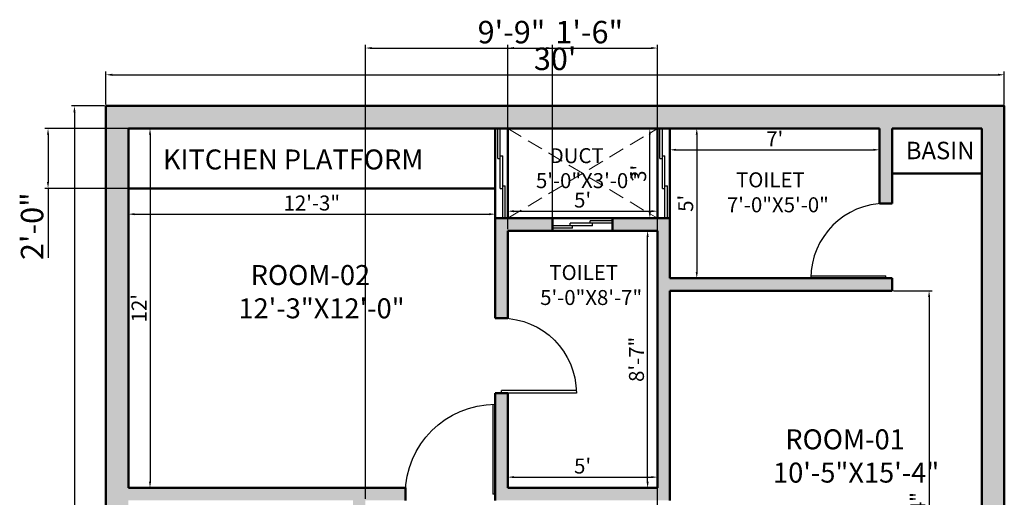
# Model space of a CAD drawing. Units: inches. Extents: x 3274 to 5176, y 1085 to 2172.
# Tile 4 of 16: x 3763 to 4158, y 1383 to 1574. Entities that reach past the tile are written whole.
import ezdxf

# ---------------------------------------------------------------- set-up
doc = ezdxf.new("R2010")
doc.units = ezdxf.units.IN
doc.linetypes.add('DASHED', pattern=[19.05, 12.7, -6.35])
for name, color, linetype, lineweight in [('A-ANNO-DIMS', 2, 'Continuous', 18), ('A-AREA-IDEN', 3, 'Continuous', 25), ('A-DOOR', 4, 'Continuous', 25), ('A-FLOR-OPEN', 7, 'DASHED', 18), ('A-GLAZ', 5, 'Continuous', 25), ('A-WALL', 7, 'Continuous', 50), ('A-WALL-PATT', 8, 'Continuous', 13)]:
    doc.layers.add(name, color=color, linetype=linetype, lineweight=lineweight)
doc.styles.get("Standard").update_dxf_attribs({"font": 'arial.ttf'})
doc.dimstyles.new('ISO-25', dxfattribs={"dimtxt": 9, "dimasz": 2.5, "dimexe": 1.25, "dimexo": 0.625, "dimtad": 1, "dimdec": 1, "dimlunit": 3, "dimtxsty": 'Standard', "dimcen": 2.5, "dimclrd": 4, "dimclre": 4, "dimclrt": 1, "dimadec": 0, "dimazin": 0, "dimtfac": 1, "dimtdec": 1, "dimtmove": 0, "dimatfit": 3, "dimfxl": 1, "dimarcsym": 0})

# ---------------------------------------------------------------- blocks, each defined once
blk = doc.blocks.new('*D8')
at = {"layer": 'A-ANNO-DIMS', "color": 0, "lineweight": -2, "transparency": 16777216}
for p, q in [((3797.7, 1539.91), (3797.7, 1553.02)), ((3800.2, 1551.77), (4155.2, 1551.77)), ((4157.7, 1539.91), (4157.7, 1553.02))]:
    blk.add_line(p, q, dxfattribs=at)
at = {"layer": 'A-ANNO-DIMS', "color": 0, "transparency": 16777216}
for points in [[(3800.2, 1552.19), (3800.2, 1551.35), (3797.7, 1551.77)], [(4155.2, 1552.19), (4155.2, 1551.35), (4157.7, 1551.77)]]:
    blk.add_solid(points, dxfattribs=at)
at = {"layer": 'Defpoints', "color": 0, "transparency": 16777216}
for p in [(4157.7, 1551.77), (3797.7, 1539.28), (4157.7, 1539.28)]:
    blk.add_point(p, dxfattribs=at)
at = {"layer": 'A-ANNO-DIMS', "color": 0, "transparency": 16777216, "insert": (3977.7, 1556.99), "char_height": 9, "attachment_point": 5}
blk.add_mtext("30'", dxfattribs=at)
blk = doc.blocks.new('*D9')
at = {"layer": 'A-ANNO-DIMS', "color": 0, "lineweight": -2, "transparency": 16777216}
for p, q in [((3797.07, 1539.28), (3783.84, 1539.28)), ((3785.09, 1536.78), (3785.09, 1181.78)), ((3797.07, 1179.28), (3783.84, 1179.28))]:
    blk.add_line(p, q, dxfattribs=at)
at = {"layer": 'A-ANNO-DIMS', "color": 0, "transparency": 16777216}
for points in [[(3784.67, 1536.78), (3785.51, 1536.78), (3785.09, 1539.28)], [(3784.67, 1181.78), (3785.51, 1181.78), (3785.09, 1179.28)]]:
    blk.add_solid(points, dxfattribs=at)
at = {"layer": 'Defpoints', "color": 0, "transparency": 16777216}
for p in [(3797.7, 1539.28), (3785.09, 1179.28), (3797.7, 1179.28)]:
    blk.add_point(p, dxfattribs=at)
at = {"layer": 'A-ANNO-DIMS', "color": 0, "transparency": 16777216, "insert": (3779.87, 1359.28), "char_height": 9, "attachment_point": 5, "rotation": 90}
blk.add_mtext("30'", dxfattribs=at)
blk = doc.blocks.new('1')
for p, q in [((0, 36), (0, 0)), ((1, 36), (1, 0)), ((0, 0), (1, 0))]:
    blk.add_line(p, q)
blk.add_arc((0, 0), 36, 0, 90)
blk = doc.blocks.new('2')
for p, q in [((0, 30), (0, 0)), ((1, 30), (1, 0)), ((0, 0), (1, 0))]:
    blk.add_line(p, q)
blk.add_arc((0, 0), 30, 0, 90)
blk = doc.blocks.new('*D34')
at = {"layer": 'A-ANNO-DIMS', "color": 0, "lineweight": -2, "transparency": 16777216}
for p, q in [((3807.32, 1530.28), (3816.62, 1530.28)), ((3815.37, 1527.78), (3815.37, 1388.78)), ((3807.32, 1386.28), (3816.62, 1386.28))]:
    blk.add_line(p, q, dxfattribs=at)
at = {"layer": 'A-ANNO-DIMS', "color": 0, "transparency": 16777216}
for points in [[(3814.96, 1527.78), (3815.79, 1527.78), (3815.37, 1530.28)], [(3814.96, 1388.78), (3815.79, 1388.78), (3815.37, 1386.28)]]:
    blk.add_solid(points, dxfattribs=at)
at = {"layer": 'Defpoints', "color": 0, "transparency": 16777216}
for p in [(3806.7, 1530.28), (3806.7, 1386.28), (3815.37, 1386.28)]:
    blk.add_point(p, dxfattribs=at)
at = {"layer": 'A-ANNO-DIMS', "color": 0, "transparency": 16777216, "insert": (3811.74, 1458.28), "char_height": 6, "attachment_point": 5, "rotation": 90}
blk.add_mtext("12'", dxfattribs=at)
blk = doc.blocks.new('*D35')
at = {"layer": 'A-ANNO-DIMS', "color": 0, "lineweight": -2, "transparency": 16777216}
for p, q in [((3806.7, 1505.66), (3806.7, 1494.69)), ((3953.7, 1505.66), (3953.7, 1494.69)), ((3809.2, 1495.94), (3951.2, 1495.94))]:
    blk.add_line(p, q, dxfattribs=at)
at = {"layer": 'A-ANNO-DIMS', "color": 0, "transparency": 16777216}
for points in [[(3809.2, 1496.35), (3809.2, 1495.52), (3806.7, 1495.94)], [(3951.2, 1496.35), (3951.2, 1495.52), (3953.7, 1495.94)]]:
    blk.add_solid(points, dxfattribs=at)
at = {"layer": 'Defpoints', "color": 0, "transparency": 16777216}
for p in [(3806.7, 1506.28), (3953.7, 1506.28), (3953.7, 1495.94)]:
    blk.add_point(p, dxfattribs=at)
at = {"layer": 'A-ANNO-DIMS', "color": 0, "transparency": 16777216, "insert": (3880.2, 1499.63), "char_height": 6, "attachment_point": 5}
blk.add_mtext('12\'-3"', dxfattribs=at)
blk = doc.blocks.new('*D47')
at = {"layer": 'A-ANNO-DIMS', "color": 0, "lineweight": -2, "transparency": 16777216}
for p, q in [((4113.32, 1465.28), (4128.81, 1465.28)), ((4127.56, 1462.78), (4127.56, 1283.78)), ((4116.82, 1281.28), (4128.81, 1281.28))]:
    blk.add_line(p, q, dxfattribs=at)
at = {"layer": 'A-ANNO-DIMS', "color": 0, "transparency": 16777216}
for points in [[(4127.15, 1462.78), (4127.98, 1462.78), (4127.56, 1465.28)], [(4127.15, 1283.78), (4127.98, 1283.78), (4127.56, 1281.28)]]:
    blk.add_solid(points, dxfattribs=at)
at = {"layer": 'Defpoints', "color": 0, "transparency": 16777216}
for p in [(4112.7, 1465.28), (4116.2, 1281.28), (4127.56, 1281.28)]:
    blk.add_point(p, dxfattribs=at)
at = {"layer": 'A-ANNO-DIMS', "color": 0, "transparency": 16777216, "insert": (4123.87, 1373.28), "char_height": 6, "attachment_point": 5, "rotation": 90}
blk.add_mtext('15\'-4"', dxfattribs=at)
blk = doc.blocks.new('*D48')
at = {"layer": 'A-ANNO-DIMS', "color": 0, "lineweight": -2, "transparency": 16777216}
for p, q in [((4023.7, 1529.66), (4023.7, 1520.47)), ((4107.7, 1529.66), (4107.7, 1520.47)), ((4026.2, 1521.72), (4105.2, 1521.72))]:
    blk.add_line(p, q, dxfattribs=at)
at = {"layer": 'A-ANNO-DIMS', "color": 0, "transparency": 16777216}
for points in [[(4026.2, 1522.14), (4026.2, 1521.3), (4023.7, 1521.72)], [(4105.2, 1522.14), (4105.2, 1521.3), (4107.7, 1521.72)]]:
    blk.add_solid(points, dxfattribs=at)
at = {"layer": 'Defpoints', "color": 0, "transparency": 16777216}
for p in [(4023.7, 1530.28), (4107.7, 1530.28), (4107.7, 1521.72)]:
    blk.add_point(p, dxfattribs=at)
at = {"layer": 'A-ANNO-DIMS', "color": 0, "transparency": 16777216, "insert": (4065.7, 1525.35), "char_height": 6, "attachment_point": 5}
blk.add_mtext("7'", dxfattribs=at)
blk = doc.blocks.new('*D49')
at = {"layer": 'A-ANNO-DIMS', "color": 0, "lineweight": -2, "transparency": 16777216}
for p, q in [((4024.32, 1530.28), (4035.71, 1530.28)), ((4034.46, 1527.78), (4034.46, 1472.78)), ((4024.32, 1470.28), (4035.71, 1470.28))]:
    blk.add_line(p, q, dxfattribs=at)
at = {"layer": 'A-ANNO-DIMS', "color": 0, "transparency": 16777216}
for points in [[(4034.05, 1527.78), (4034.88, 1527.78), (4034.46, 1530.28)], [(4034.05, 1472.78), (4034.88, 1472.78), (4034.46, 1470.28)]]:
    blk.add_solid(points, dxfattribs=at)
at = {"layer": 'Defpoints', "color": 0, "transparency": 16777216}
for p in [(4023.7, 1530.28), (4023.7, 1470.28), (4034.46, 1470.28)]:
    blk.add_point(p, dxfattribs=at)
at = {"layer": 'A-ANNO-DIMS', "color": 0, "transparency": 16777216, "insert": (4030.79, 1500.28), "char_height": 6, "attachment_point": 5, "rotation": 90}
blk.add_mtext("5'", dxfattribs=at)
blk = doc.blocks.new('*D50')
at = {"layer": 'A-ANNO-DIMS', "color": 0, "lineweight": -2, "transparency": 16777216}
for p, q in [((3958.7, 1494.91), (3958.7, 1498.38)), ((3961.2, 1497.13), (4016.2, 1497.13)), ((4018.7, 1494.91), (4018.7, 1498.38))]:
    blk.add_line(p, q, dxfattribs=at)
at = {"layer": 'A-ANNO-DIMS', "color": 0, "transparency": 16777216}
for points in [[(3961.2, 1497.55), (3961.2, 1496.71), (3958.7, 1497.13)], [(4016.2, 1497.55), (4016.2, 1496.71), (4018.7, 1497.13)]]:
    blk.add_solid(points, dxfattribs=at)
at = {"layer": 'Defpoints', "color": 0, "transparency": 16777216}
for p in [(4018.7, 1497.13), (3958.7, 1494.28), (4018.7, 1494.28)]:
    blk.add_point(p, dxfattribs=at)
at = {"layer": 'A-ANNO-DIMS', "color": 0, "transparency": 16777216, "insert": (3988.7, 1500.81), "char_height": 6, "attachment_point": 5}
blk.add_mtext("5'", dxfattribs=at)
blk = doc.blocks.new('*D51')
at = {"layer": 'A-ANNO-DIMS', "color": 0, "lineweight": -2, "transparency": 16777216}
for p, q in [((4018.07, 1530.28), (4014.39, 1530.28)), ((4015.64, 1496.78), (4015.64, 1527.78)), ((4018.07, 1494.28), (4014.39, 1494.28))]:
    blk.add_line(p, q, dxfattribs=at)
at = {"layer": 'A-ANNO-DIMS', "color": 0, "transparency": 16777216}
for points in [[(4015.22, 1527.78), (4016.06, 1527.78), (4015.64, 1530.28)], [(4015.22, 1496.78), (4016.06, 1496.78), (4015.64, 1494.28)]]:
    blk.add_solid(points, dxfattribs=at)
at = {"layer": 'Defpoints', "color": 0, "transparency": 16777216}
for p in [(4015.64, 1530.28), (4018.7, 1530.28), (4018.7, 1494.28)]:
    blk.add_point(p, dxfattribs=at)
at = {"layer": 'A-ANNO-DIMS', "color": 0, "transparency": 16777216, "insert": (4011.95, 1512.28), "char_height": 6, "attachment_point": 5, "rotation": 90}
blk.add_mtext("3'", dxfattribs=at)
blk = doc.blocks.new('*D52')
at = {"layer": 'A-ANNO-DIMS', "color": 0, "lineweight": -2, "transparency": 16777216}
for p, q in [((3958.7, 1386.91), (3958.7, 1391.85)), ((3961.2, 1390.6), (4016.2, 1390.6)), ((4018.7, 1386.91), (4018.7, 1391.85))]:
    blk.add_line(p, q, dxfattribs=at)
at = {"layer": 'A-ANNO-DIMS', "color": 0, "transparency": 16777216}
for points in [[(3961.2, 1391.02), (3961.2, 1390.19), (3958.7, 1390.6)], [(4016.2, 1391.02), (4016.2, 1390.19), (4018.7, 1390.6)]]:
    blk.add_solid(points, dxfattribs=at)
at = {"layer": 'Defpoints', "color": 0, "transparency": 16777216}
for p in [(4018.7, 1390.6), (3958.7, 1386.28), (4018.7, 1386.28)]:
    blk.add_point(p, dxfattribs=at)
at = {"layer": 'A-ANNO-DIMS', "color": 0, "transparency": 16777216, "insert": (3988.7, 1394.28), "char_height": 6, "attachment_point": 5}
blk.add_mtext("5'", dxfattribs=at)
blk = doc.blocks.new('*D53')
at = {"layer": 'A-ANNO-DIMS', "color": 0, "lineweight": -2, "transparency": 16777216}
for p, q in [((4018.07, 1489.28), (4013.51, 1489.28)), ((4014.76, 1388.78), (4014.76, 1486.78)), ((4018.07, 1386.28), (4013.51, 1386.28))]:
    blk.add_line(p, q, dxfattribs=at)
at = {"layer": 'A-ANNO-DIMS', "color": 0, "transparency": 16777216}
for points in [[(4014.34, 1486.78), (4015.18, 1486.78), (4014.76, 1489.28)], [(4014.34, 1388.78), (4015.18, 1388.78), (4014.76, 1386.28)]]:
    blk.add_solid(points, dxfattribs=at)
at = {"layer": 'Defpoints', "color": 0, "transparency": 16777216}
for p in [(4014.76, 1489.28), (4018.7, 1489.28), (4018.7, 1386.28)]:
    blk.add_point(p, dxfattribs=at)
at = {"layer": 'A-ANNO-DIMS', "color": 0, "transparency": 16777216, "insert": (4011.07, 1437.78), "char_height": 6, "attachment_point": 5, "rotation": 90}
blk.add_mtext('8\'-7"', dxfattribs=at)
blk = doc.blocks.new('WIN-24')
for p, q in [((4552.19, 1485.35), (4536.19, 1485.35)), ((4544.19, 1484.35), (4536.19, 1484.35)), ((4560.19, 1486.35), (4543.19, 1486.35)), ((4543.19, 1485.35), (4543.19, 1486.35)), ((4544.19, 1484.35), (4544.19, 1485.35)), ((4551.19, 1486.35), (4551.19, 1487.35)), ((4560.19, 1487.35), (4551.19, 1487.35)), ((4552.19, 1485.35), (4552.19, 1486.35))]:
    blk.add_line(p, q)
blk = doc.blocks.new('WIN-36')
for p, q in [((4514.19, 1512.35), (4514.19, 1524.35)), ((4515.19, 1500.35), (4515.19, 1524.35)), ((4514.19, 1512.35), (4515.19, 1512.35)), ((4515.19, 1513.35), (4516.19, 1513.35)), ((4516.19, 1488.35), (4516.19, 1513.35)), ((4515.19, 1500.35), (4516.19, 1500.35)), ((4516.19, 1501.35), (4517.19, 1501.35)), ((4517.19, 1488.35), (4517.19, 1501.35))]:
    blk.add_line(p, q)
blk = doc.blocks.new('*D196')
at = {"layer": 'A-ANNO-DIMS', "color": 4, "lineweight": -2, "transparency": 16777216}
for p, q in [((3953.07, 1530.28), (3773.25, 1530.28)), ((3774.5, 1527.78), (3774.5, 1508.78)), ((3953.07, 1506.28), (3773.25, 1506.28)), ((3774.5, 1506.28), (3774.5, 1478.45))]:
    blk.add_line(p, q, dxfattribs=at)
at = {"layer": 'A-ANNO-DIMS', "color": 4, "transparency": 16777216}
for points in [[(3774.08, 1527.78), (3774.91, 1527.78), (3774.5, 1530.28)], [(3774.08, 1508.78), (3774.91, 1508.78), (3774.5, 1506.28)]]:
    blk.add_solid(points, dxfattribs=at)
at = {"layer": 'Defpoints', "color": 0, "transparency": 16777216}
for p in [(3953.7, 1530.28), (3774.5, 1506.28), (3953.7, 1506.28)]:
    blk.add_point(p, dxfattribs=at)
at = {"layer": 'A-ANNO-DIMS', "color": 1, "transparency": 16777216, "insert": (3769.27, 1491.12), "char_height": 9, "attachment_point": 5, "rotation": 90}
blk.add_mtext('2\'-0"', dxfattribs=at)
blk = doc.blocks.new('*D200')
at = {"layer": 'A-ANNO-DIMS', "color": 4, "lineweight": -2, "transparency": 16777216}
for p, q in [((3901.7, 1381.91), (3901.7, 1563.73)), ((3904.2, 1562.48), (4016.2, 1562.48)), ((4018.7, 1345.91), (4018.7, 1563.73))]:
    blk.add_line(p, q, dxfattribs=at)
at = {"layer": 'A-ANNO-DIMS', "color": 4, "transparency": 16777216}
for points in [[(3904.2, 1562.9), (3904.2, 1562.06), (3901.7, 1562.48)], [(4016.2, 1562.9), (4016.2, 1562.06), (4018.7, 1562.48)]]:
    blk.add_solid(points, dxfattribs=at)
at = {"layer": 'Defpoints', "color": 0, "transparency": 16777216}
for p in [(4018.7, 1562.48), (3901.7, 1381.28), (4018.7, 1345.28)]:
    blk.add_point(p, dxfattribs=at)
at = {"layer": 'A-ANNO-DIMS', "color": 1, "transparency": 16777216, "insert": (3960.2, 1567.7), "char_height": 9, "attachment_point": 5}
blk.add_mtext('9\'-9"', dxfattribs=at)
blk = doc.blocks.new('*D203')
at = {"layer": 'A-ANNO-DIMS', "color": 4, "lineweight": -2, "transparency": 16777216}
for p, q in [((3958.7, 1489.91), (3958.7, 1563.73)), ((3961.2, 1562.48), (3974.2, 1562.48)), ((3976.7, 1489.91), (3976.7, 1563.73)), ((3976.7, 1562.48), (4003.52, 1562.48))]:
    blk.add_line(p, q, dxfattribs=at)
at = {"layer": 'A-ANNO-DIMS', "color": 4, "transparency": 16777216}
for points in [[(3961.2, 1562.9), (3961.2, 1562.06), (3958.7, 1562.48)], [(3974.2, 1562.9), (3974.2, 1562.06), (3976.7, 1562.48)]]:
    blk.add_solid(points, dxfattribs=at)
at = {"layer": 'Defpoints', "color": 0, "transparency": 16777216}
for p in [(3976.7, 1562.48), (3958.7, 1489.28), (3976.7, 1489.28)]:
    blk.add_point(p, dxfattribs=at)
at = {"layer": 'A-ANNO-DIMS', "color": 1, "transparency": 16777216, "insert": (3991.36, 1567.7), "char_height": 9, "attachment_point": 5}
blk.add_mtext('1\'-6"', dxfattribs=at)

msp = doc.modelspace()

# ---------------------------------------------------------------- hatches: boundary and pattern name
at = {"layer": 'A-WALL-PATT'}
h = msp.add_hatch(color=256, dxfattribs=at)
h.dxf.hatch_style = 1
h.paths.add_polyline_path([(3958.7, 1489.28), (3976.7, 1489.28), (3976.7, 1494.28), (3953.7, 1494.28), (3953.7, 1454.28), (3958.7, 1454.28)], flags=17)
h.paths.add_polyline_path([(4023.7, 1494.28), (4000.7, 1494.28), (4000.7, 1489.28), (4018.7, 1489.28), (4018.7, 1386.28), (3958.7, 1386.28), (3958.7, 1424.28), (3956.2, 1424.28), (3953.7, 1424.28), (3953.7, 1381.28), (4023.7, 1381.28), (4023.7, 1465.28), (4112.7, 1465.28), (4112.7, 1470.28), (4023.7, 1470.28)], flags=17)
h.paths.add_polyline_path([(4056.2, 1281.28), (4023.7, 1281.28), (4023.7, 1345.28), (4018.7, 1345.28), (4018.7, 1281.28), (4011.7, 1281.28), (4011.7, 1276.78), (4011.7, 1272.28), (4056.2, 1272.28)], flags=17)
h.paths.add_polyline_path([(3963.7, 1281.28), (3958.7, 1281.28), (3958.7, 1325.28), (3953.7, 1325.28), (3953.7, 1188.28), (3902.7, 1188.28), (3902.7, 1179.28), (3958.7, 1179.28), (3958.7, 1272.28), (3963.7, 1272.28)], flags=17)
h.paths.add_polyline_path([(3806.7, 1530.28), (4107.7, 1530.28), (4107.7, 1500.28), (4112.7, 1500.28), (4112.7, 1530.28), (4148.7, 1530.28), (4148.7, 1281.28), (4116.2, 1281.28), (4116.2, 1272.28), (4148.7, 1272.28), (4148.7, 1188.28), (4106.7, 1188.28), (4106.7, 1179.28), (4157.7, 1179.28), (4157.7, 1539.28), (3797.7, 1539.28), (3797.7, 1179.28), (3830.7, 1179.28), (3830.7, 1188.28), (3806.7, 1188.28), (3806.7, 1381.28), (3896.7, 1381.28), (3896.7, 1320.28), (3917.7, 1320.28), (3917.7, 1325.28), (3901.7, 1325.28), (3901.7, 1381.28), (3917.7, 1381.28), (3917.7, 1386.28), (3806.7, 1386.28)])
h.paths.add_polyline_path([(3866.7, 1325.28), (3841.7, 1325.28), (3841.7, 1345.28), (3836.7, 1345.28), (3836.7, 1320.28), (3866.7, 1320.28)], flags=17)
h.paths.add_polyline_path([(4115.78, 1513.99), (4148.63, 1513.99), (4148.63, 1528.42), (4115.78, 1528.42)], flags=25)
h.paths.add_polyline_path([(3961.09, 1219.59), (4026.99, 1219.59), (4026.99, 1252.09), (3961.09, 1252.09)], flags=25)
h.paths.add_polyline_path([(3956.63, 1343.39), (3997.9, 1343.39), (3997.9, 1359.88), (3956.63, 1359.88)], flags=25)
h.paths.add_polyline_path([(3817.73, 1191.34), (3934.74, 1191.34), (3934.74, 1207.83), (3817.73, 1207.83)], flags=25)
h.paths.add_polyline_path([(3817.73, 1509.34), (3934.74, 1509.34), (3934.74, 1525.83), (3817.73, 1525.83)], flags=25)
h.paths.add_polyline_path([(4061.81, 1383.87), (4130.2, 1383.87), (4130.2, 1413.72), (4061.81, 1413.72)], flags=25)
h.paths.add_polyline_path([(3847.58, 1243.23), (3915.98, 1243.23), (3915.98, 1273.08), (3847.58, 1273.08)], flags=25)
h.paths.add_polyline_path([(4044.62, 1493.29), (4086.59, 1493.29), (4086.59, 1515.68), (4044.62, 1515.68)], flags=25)
h.paths.add_polyline_path([(3968.18, 1502.97), (4010.15, 1502.97), (4010.15, 1525.36), (3968.18, 1525.36)], flags=25)
h.paths.add_polyline_path([(3969.86, 1456.15), (4011.83, 1456.15), (4011.83, 1478.54), (3969.86, 1478.54)], flags=24)
h.paths.add_polyline_path([(3847.58, 1449.68), (3915.98, 1449.68), (3915.98, 1479.54), (3847.58, 1479.54)], flags=25)
h.paths.add_polyline_path([(4019.88, 1246.5), (4034.58, 1246.5), (4034.58, 1255.65), (4019.88, 1255.65)], flags=25)
h.paths.add_polyline_path([(4019.91, 1204.63), (4035.01, 1204.63), (4035.01, 1213.63), (4019.91, 1213.63)], flags=25)
h.paths.add_polyline_path([(3825.87, 1349.35), (3867.84, 1349.35), (3867.84, 1371.74), (3825.87, 1371.74)], flags=25)

# ---------------------------------------------------------------- linework, layer by layer
at = {"layer": 'A-FLOR-OPEN', "ltscale": 0.5}
for p, q in [((3958.7, 1530.28), (4018.7, 1494.28)), ((3958.7, 1494.28), (4018.7, 1530.28))]:
    msp.add_line(p, q, dxfattribs=at)
at = {"layer": 'A-WALL'}
for p, q in [((3806.7, 1530.28), (4107.7, 1530.28)), ((3806.7, 1386.28), (3806.7, 1530.28)), ((3953.7, 1454.28), (3953.7, 1530.28)), ((3958.7, 1494.28), (3958.7, 1530.28)), ((4018.7, 1530.28), (4018.7, 1494.28)), ((4023.7, 1530.28), (4023.7, 1470.28)), ((4107.7, 1530.28), (4107.7, 1500.28)), ((4112.7, 1530.28), (4148.7, 1530.28)), ((4112.7, 1530.28), (4112.7, 1500.28)), ((4148.7, 1530.28), (4148.7, 1281.28)), ((4112.7, 1512.28), (4148.7, 1512.28)), ((3806.7, 1506.28), (3953.7, 1506.28)), ((4107.7, 1500.28), (4112.7, 1500.28)), ((3953.7, 1494.28), (4023.7, 1494.28)), ((3976.7, 1489.28), (3976.7, 1494.28)), ((4000.7, 1489.28), (4000.7, 1494.28)), ((3958.7, 1489.28), (4018.7, 1489.28)), ((3958.7, 1454.28), (3958.7, 1489.28)), ((4018.7, 1489.28), (4018.7, 1386.28)), ((4023.7, 1470.28), (4112.7, 1470.28)), ((4112.7, 1470.28), (4112.7, 1465.28)), ((4023.7, 1465.28), (4112.7, 1465.28)), ((4023.7, 1465.28), (4023.7, 1381.28)), ((3953.7, 1454.28), (3958.7, 1454.28)), ((3953.7, 1424.28), (3958.7, 1424.28)), ((3953.7, 1381.28), (3953.7, 1424.28)), ((3958.7, 1386.28), (3958.7, 1424.28)), ((3806.7, 1386.28), (3917.7, 1386.28)), ((3917.7, 1381.28), (3917.7, 1386.28)), ((3958.7, 1386.28), (4018.7, 1386.28))]:
    msp.add_line(p, q, dxfattribs=at)
msp.add_lwpolyline([(3958.7, 1179.28), (3797.7, 1179.28), (3797.7, 1539.28), (4157.7, 1539.28), (4157.7, 1179.28), (3958.7, 1179.28)], dxfattribs=at)

# ---------------------------------------------------------------- block references
at = {"layer": 'A-DOOR', "rotation": 89.99999999999999}
msp.add_blockref('2', (4110.2, 1470.28), dxfattribs=at)
at = {"layer": 'A-DOOR', "xscale": -1, "rotation": 270}
msp.add_blockref('2', (3956.2, 1424.28), dxfattribs=at)
at = {"layer": 'A-DOOR', "xscale": -1}
msp.add_blockref('1', (3953.7, 1383.78), dxfattribs=at)
at = {"layer": 'A-GLAZ'}
for name, p in [('WIN-36', (-559.49, 5.93)), ('WIN-36', (-494.49, 5.93)), ('WIN-24', (-559.49, 5.93))]:
    msp.add_blockref(name, p, dxfattribs=at)

# ---------------------------------------------------------------- texts
at = {"layer": 'A-AREA-IDEN', "attachment_point": 1}
for s, width, heights, insert, char_height in [('BASIN', 147.1149, [0], (4118.25, 1524.94), 7), ('KITCHEN PLATFORM', 147.1149, [0], (3820.54, 1521.85), 8), ('   DUCT\\P5\'-0"X3\'-0"', 58.0121, [16.24], (3970.02, 1522.37), 6), ('  TOILET\\P7\'-0"X5\'-0"', 58.0121, [16.24], (4046.52, 1512.7), 6), ('  ROOM-02\\P12\'-3"X12\'-0"', 58.0121, [0], (3850.8, 1475.56), 8), ('  TOILET\\P5\'-0"X8\'-7"', 58.0121, [16.24], (3971.71, 1475.56), 6), ('  ROOM-01\\P10\'-5"X15\'-4"', 58.0121, [0], (4065.03, 1409.75), 8)]:
    msp.add_mtext_dynamic_manual_height_columns(s, width=width, gutter_width=30, heights=heights, dxfattribs=dict(at, insert=insert, char_height=char_height))

# ---------------------------------------------------------------- dimensions: what is measured, and where the dimension line sits
at = {"layer": 'A-ANNO-DIMS'}
for base, p1, p2, override, picture, middle in [((4018.7, 1562.48), (3901.7, 1381.28), (4018.7, 1345.28), {"dimdec": 1, "dimlfac": 1, "dimrnd": 0, "dimzin": 1, "dimdsep": 46, "dimlunit": 4, "dimfrac": 2}, '*D200', (3960.2, 1567.7)), ((3976.7, 1562.48), (3958.7, 1489.28), (3976.7, 1489.28), {"dimdec": 1, "dimlfac": 1, "dimrnd": 0, "dimzin": 1, "dimdsep": 46, "dimlunit": 4, "dimfrac": 2}, '*D203', (3991.36, 1567.7)), ((4157.7, 1551.77), (3797.7, 1539.28), (4157.7, 1539.28), {"dimclrd": 0, "dimclre": 0, "dimclrt": 0}, '*D8', (3977.7, 1556.99)), ((4107.7, 1521.72), (4023.7, 1530.28), (4107.7, 1530.28), {"dimtxt": 6, "dimclrd": 0, "dimclre": 0, "dimclrt": 0}, '*D48', (4065.7, 1525.35)), ((3953.7, 1495.94), (3806.7, 1506.28), (3953.7, 1506.28), {"dimtxt": 6, "dimclrd": 0, "dimclre": 0, "dimclrt": 0}, '*D35', (3880.2, 1499.63)), ((4018.7, 1497.13), (3958.7, 1494.28), (4018.7, 1494.28), {"dimtxt": 6, "dimclrd": 0, "dimclre": 0, "dimclrt": 0}, '*D50', (3988.7, 1500.81)), ((4018.7, 1390.6), (3958.7, 1386.28), (4018.7, 1386.28), {"dimtxt": 6, "dimclrd": 0, "dimclre": 0, "dimclrt": 0}, '*D52', (3988.7, 1394.28))]:
    dim = msp.add_linear_dim(base=base, p1=p1, p2=p2, dimstyle='ISO-25', override=override, dxfattribs=at)
    dim.commit()
    dim.dimension.update_dxf_attribs({"geometry": picture, "text_midpoint": middle})
for base, p1, p2, override, picture, middle in [((3785.09, 1179.28), (3797.7, 1539.28), (3797.7, 1179.28), {"dimclrd": 0, "dimclre": 0, "dimclrt": 0}, '*D9', (3779.87, 1359.28)), ((3774.5, 1506.28), (3953.7, 1530.28), (3953.7, 1506.28), {"dimdec": 1, "dimlfac": 1, "dimrnd": 0, "dimzin": 1, "dimdsep": 46, "dimlunit": 4, "dimfrac": 2}, '*D196', (3769.27, 1491.12)), ((3815.37, 1386.28), (3806.7, 1530.28), (3806.7, 1386.28), {"dimtxt": 6, "dimclrd": 0, "dimclre": 0, "dimclrt": 0}, '*D34', (3811.74, 1458.28)), ((4015.64, 1530.28), (4018.7, 1494.28), (4018.7, 1530.28), {"dimtxt": 6, "dimclrd": 0, "dimclre": 0, "dimclrt": 0}, '*D51', (4011.95, 1512.28)), ((4034.46, 1470.28), (4023.7, 1530.28), (4023.7, 1470.28), {"dimtxt": 6, "dimclrd": 0, "dimclre": 0, "dimclrt": 0}, '*D49', (4030.79, 1500.28)), ((4014.76, 1489.28), (4018.7, 1386.28), (4018.7, 1489.28), {"dimtxt": 6, "dimclrd": 0, "dimclre": 0, "dimclrt": 0}, '*D53', (4011.07, 1437.78)), ((4127.56, 1281.28), (4112.7, 1465.28), (4116.2, 1281.28), {"dimtxt": 6, "dimclrd": 0, "dimclre": 0, "dimclrt": 0}, '*D47', (4123.87, 1373.28))]:
    dim = msp.add_linear_dim(base=base, p1=p1, p2=p2, angle=90, dimstyle='ISO-25', override=override, dxfattribs=at)
    dim.commit()
    dim.dimension.update_dxf_attribs({"geometry": picture, "text_midpoint": middle})

doc.saveas('drawing.dxf')
